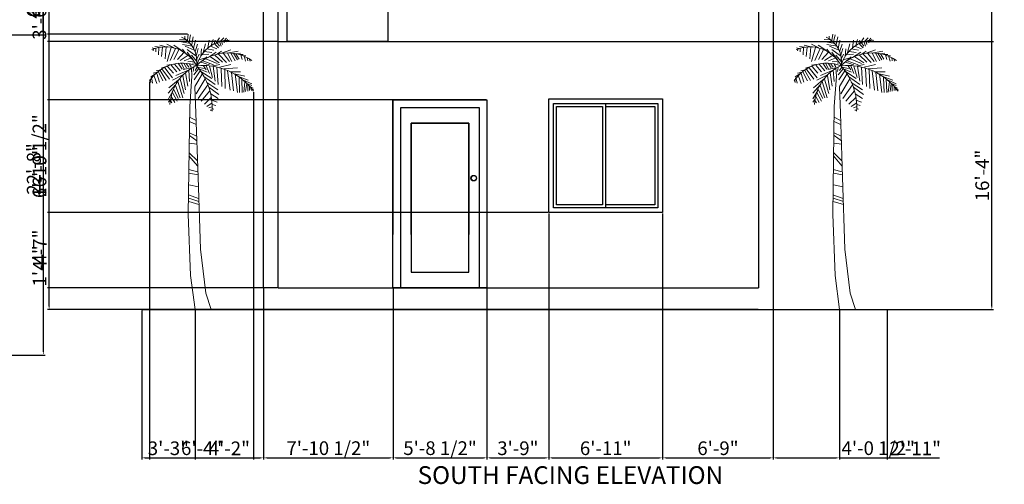
# Model space of a CAD drawing. Units: inches. Extents: x 1344 to 2521, y 3236 to 4924.
# Tile 13 of 14: x 1801 to 2521, y 4059 to 4398. Entities that reach past the tile are written whole.
import ezdxf

# ---------------------------------------------------------------- set-up
doc = ezdxf.new("R2010")
doc.units = ezdxf.units.IN
for name, color, linetype, lineweight in [('A-ANNO-DIMS', 2, 'Continuous', 18), ('A-ANNO-TEXT', 7, 'Continuous', 25), ('A-DOOR', 50, 'Continuous', 25), ('A-ELEV', 7, 'Continuous', 25), ('A-GLAZ', 150, 'Continuous', 25), ('L-PLNT', 82, 'Continuous', 13)]:
    doc.layers.add(name, color=color, linetype=linetype, lineweight=lineweight)
doc.styles.get("Standard").update_dxf_attribs({"font": 'arial.ttf'})
doc.dimstyles.new('ISO-25', dxfattribs={"dimtxt": 10, "dimasz": 2.5, "dimexe": 1.25, "dimexo": 0.625, "dimtad": 1, "dimdec": 0, "dimlunit": 4, "dimtxsty": 'Standard', "dimcen": 2.5, "dimadec": 0, "dimazin": 0, "dimtfac": 1, "dimtdec": 0, "dimtmove": 0, "dimatfit": 3, "dimfxl": 1, "dimarcsym": 0})

# ---------------------------------------------------------------- blocks, each defined once
blk = doc.blocks.new('*U10')
for p, q in [((1.5, 1.5), (1.5, 34.5)), ((1.5, 34.5), (18, 34.5)), ((18, 1.5), (18, 34.5)), ((18, 34.5), (34.5, 34.5)), ((34.5, 34.5), (34.5, 1.5)), ((18, 1.5), (1.5, 1.5)), ((34.5, 1.5), (18, 1.5))]:
    blk.add_line(p, q)
blk.add_lwpolyline([(0, 0), (0, 36), (36, 36), (36, 0)], close=True)
for points in [[(17, 33.5), (17, 2.5), (2.5, 2.5), (2.5, 33.5), (17, 33.5)], [(18, 33.5), (33.5, 33.5), (33.5, 2.5), (18, 2.5)]]:
    blk.add_lwpolyline(points)
blk = doc.blocks.new('*U13')
blk.add_lwpolyline([(3.12, 0.01), (0.12, 0.01), (0.12, 72.01), (36.12, 72.01), (36.12, 0.01), (33.12, 0.01)])
for points in [[(33.12, 68.99), (33.12, 0.01), (3.12, 0.01), (3.12, 68.99)], [(29.12, 6.01), (29.12, 62.99), (7.12, 62.99), (7.12, 6.01)]]:
    blk.add_lwpolyline(points, close=True)
blk.add_circle((31.12, 42.01), 1)
blk = doc.blocks.new('*U14')
for p, q in [((-6.727, 197.202), (-11.366, 197.45)), ((-3.441, 194.477), (-10.013, 195.716)), ((-7.5, 199.68), (-7.5, 197.946)), ((-5.567, 196.707), (-4.987, 201.167)), ((-4.407, 195.716), (-3.247, 200.672)), ((-2.474, 193.733), (-1.315, 199.433)), ((-1.121, 190.759), (0.232, 196.955)), ((9.317, 191.255), (10.283, 196.955)), ((11.829, 192.99), (13.182, 197.45)), ((13.956, 194.229), (14.729, 196.955)), ((15.116, 194.477), (17.822, 198.689)), ((16.082, 194.972), (17.822, 192.494)), ((18.015, 195.716), (20.914, 198.689)), ((18.015, 195.468), (18.981, 192.494)), ((19.368, 196.459), (19.948, 193.733)), ((20.914, 196.459), (21.301, 194.972)), ((21.301, 196.459), (22.847, 198.441)), ((22.074, 196.707), (23.427, 195.716)), ((23.234, 196.707), (23.62, 197.698)), ((-29.729, 190.759), (-31.469, 191.255)), ((-30.309, 190.512), (-30.695, 189.025)), ((-25.283, 191.751), (-29.342, 192.246)), ((-28.763, 190.759), (-28.763, 188.281)), ((-26.443, 191.503), (-26.636, 186.051)), ((-20.064, 191.751), (-25.863, 193.238)), ((-23.737, 191.751), (-24.51, 185.06)), ((-21.031, 191.998), (-21.804, 183.325)), ((-15.232, 191.255), (-20.644, 193.981)), ((-17.551, 191.503), (-20.451, 181.343)), ((-14.265, 190.759), (-18.131, 182.086)), ((-9.433, 189.025), (-15.618, 193.238)), ((-11.753, 189.768), (-15.425, 182.83)), ((-8.08, 188.034), (-12.912, 182.83)), ((-1.894, 192.494), (-9.24, 193.733)), ((-6.147, 186.299), (-9.24, 190.264)), ((-0.541, 189.52), (-7.307, 192.494)), ((-5.76, 190.016), (0.618, 185.308)), ((-5.76, 188.034), (-1.508, 182.582)), ((0.038, 188.281), (1.778, 193.981)), ((1.005, 185.803), (2.358, 190.759)), ((4.098, 185.06), (4.678, 190.512)), ((5.837, 187.786), (7.577, 194.229)), ((6.997, 188.529), (12.216, 187.786)), ((8.544, 190.512), (13.763, 189.52)), ((9.51, 184.317), (15.502, 188.034)), ((11.25, 192.494), (15.889, 190.512)), ((14.536, 193.981), (17.242, 191.255)), ((15.695, 186.299), (19.368, 188.777)), ((19.368, 187.29), (26.133, 189.768)), ((23.814, 187.29), (26.907, 181.343)), ((24.78, 187.538), (31.546, 188.777)), ((26.133, 187.29), (29.419, 181.838)), ((28.066, 187.29), (30.966, 182.582)), ((29.999, 186.795), (33.092, 187.29)), ((-12.332, 180.104), (-9.433, 175.643)), ((-4.987, 185.803), (-10.979, 182.086)), ((-10.206, 180.104), (-8.08, 175.891)), ((-8.273, 180.104), (-6.147, 176.635)), ((-3.247, 183.821), (-8.08, 181.838)), ((-1.315, 181.591), (-5.374, 181.095)), ((-2.668, 185.803), (1.198, 181.343)), ((-0.348, 180.352), (-1.894, 180.104)), ((1.005, 182.582), (2.938, 186.547)), ((2.938, 182.582), (6.61, 183.821)), ((4.098, 180.847), (8.35, 179.608)), ((4.871, 186.051), (10.09, 186.547)), ((4.871, 181.591), (8.544, 184.812)), ((5.644, 181.838), (13.569, 178.865)), ((7.77, 183.325), (16.082, 179.856)), ((11.25, 184.812), (17.628, 180.352)), ((14.536, 185.803), (19.948, 180.847)), ((17.242, 186.547), (23.041, 180.599)), ((20.721, 187.042), (25.167, 181.343)), ((29.806, 186.795), (32.319, 183.078)), ((32.512, 186.299), (35.218, 186.299)), ((33.479, 186.051), (34.445, 182.83)), ((35.605, 185.556), (37.151, 185.308)), ((35.798, 185.308), (36.958, 181.591)), ((38.118, 184.317), (38.504, 181.838)), ((39.857, 182.83), (40.244, 181.591)), ((-27.409, 173.413), (-30.695, 172.67)), ((-25.09, 175.148), (-28.376, 174.404)), ((-26.829, 173.661), (-23.544, 167.218)), ((-25.476, 174.652), (-21.224, 167.466)), ((-21.031, 177.626), (-24.897, 176.387)), ((-24.317, 175.891), (-18.711, 168.457)), ((-22.191, 176.635), (-16.391, 169.448)), ((-15.618, 179.36), (-20.644, 178.617)), ((-20.064, 177.626), (-15.812, 172.67)), ((-17.358, 178.617), (-13.299, 173.661)), ((-15.038, 179.36), (-10.786, 174.404)), ((-4.214, 175.148), (-14.072, 170.935)), ((-1.701, 176.882), (-8.66, 175.396)), ((-6.92, 172.917), (-5.374, 163.253)), ((-6.34, 179.608), (-4.6, 177.13)), ((-4.6, 174.9), (-4.021, 166.722)), ((-4.021, 179.36), (-2.861, 177.378)), ((-2.668, 176.387), (-2.376, 170.594)), ((-0.928, 176.882), (-1.508, 173.909)), ((2.551, 175.891), (-0.928, 171.431)), ((3.711, 174.404), (-0.541, 167.961)), ((1.585, 177.13), (0.038, 174.652)), ((1.585, 177.13), (6.61, 176.139)), ((2.938, 175.891), (8.737, 173.413)), ((4.291, 173.909), (12.216, 168.953)), ((6.224, 178.121), (8.157, 175.148)), ((7.384, 178.369), (10.476, 179.36)), ((8.157, 178.121), (10.476, 172.422)), ((10.476, 177.874), (12.796, 169.696)), ((11.829, 177.874), (18.015, 179.113)), ((13.182, 177.874), (14.729, 166.97)), ((15.889, 177.13), (16.855, 164.492)), ((18.015, 177.13), (26.133, 179.113)), ((18.981, 175.891), (19.561, 163.005)), ((20.914, 175.891), (30.966, 176.635)), ((21.688, 175.396), (22.074, 161.518)), ((23.814, 174.404), (25.554, 160.279)), ((25.554, 173.661), (33.285, 173.661)), ((26.52, 173.165), (28.066, 159.784)), ((-32.628, 167.961), (-33.208, 167.961)), ((-32.628, 167.713), (-32.435, 165.979)), ((-28.956, 172.174), (-32.435, 170.192)), ((-31.082, 169.944), (-32.435, 169.2)), ((-31.662, 168.705), (-31.082, 165.483)), ((-29.922, 170.687), (-27.989, 165.235)), ((-27.989, 172.422), (-26.056, 166.227)), ((-12.139, 167.961), (-19.098, 162.014)), ((-8.466, 171.678), (-16.585, 167.713)), ((-12.719, 166.722), (-9.046, 154.828)), ((-10.979, 168.457), (-7.887, 157.801)), ((-8.853, 170.935), (-7.113, 160.527)), ((5.257, 171.926), (-0.155, 163.005)), ((7.384, 168.705), (0.812, 157.553)), ((6.417, 170.439), (14.729, 164.492)), ((8.544, 165.979), (16.662, 160.527)), ((28.839, 172.174), (36.378, 170.687)), ((29.226, 171.926), (30.966, 158.545)), ((30.966, 170.687), (38.891, 167.713)), ((32.126, 169.696), (32.512, 158.545)), ((34.058, 168.705), (34.445, 158.545)), ((35.412, 167.713), (41.404, 164.988)), ((36.378, 166.474), (35.605, 158.792)), ((-14.265, 164.244), (-19.678, 158.049)), ((-16.005, 160.031), (-19.484, 154.084)), ((-16.585, 158.545), (-13.106, 152.35)), ((-15.618, 160.775), (-12.332, 154.332)), ((-14.265, 163.749), (-10.786, 154.828)), ((9.317, 164.244), (2.358, 154.332)), ((10.863, 159.784), (4.484, 152.35)), ((10.09, 162.51), (17.435, 157.058)), ((37.731, 165.235), (36.958, 159.288)), ((37.924, 165.235), (41.404, 163.749)), ((38.504, 164.492), (38.504, 159.536)), ((39.664, 163.253), (42.37, 161.766)), ((39.857, 162.757), (39.857, 160.031)), ((40.824, 161.766), (41.21, 160.031)), ((41.21, 161.518), (42.757, 160.279)), ((-18.131, 153.589), (-19.484, 151.606)), ((-17.938, 152.597), (-16.972, 151.111)), ((-17.358, 155.819), (-14.845, 151.358)), ((11.829, 155.075), (6.804, 150.119)), ((11.443, 157.553), (16.855, 154.332)), ((12.216, 153.093), (16.082, 151.606)), ((12.603, 151.111), (8.544, 148.385)), ((12.216, 148.137), (10.09, 147.393)), ((12.409, 145.659), (11.056, 145.659)), ((12.409, 146.898), (13.763, 146.402)), ((12.603, 149.872), (15.116, 149.128)), ((-4.081, 140.645), (0.753, 138.261)), ((-4.081, 137.547), (0.753, 135.163)), ((-4.081, 129.205), (1.124, 126.821)), ((-4.081, 127.298), (1.31, 123.246)), ((-4.081, 121.578), (1.31, 120.863)), ((-4.453, 112.283), (1.682, 105.133)), ((-4.267, 114.428), (1.682, 108.708)), ((-4.639, 102.273), (1.868, 100.604)), ((-4.453, 99.651), (2.24, 98.459)), ((-4.453, 91.071), (2.426, 89.641)), ((-4.825, 83.921), (2.612, 81.061)), ((-4.639, 81.299), (2.797, 78.916)), ((-4.639, 78.916), (2.797, 76.771))]:
    blk.add_line(p, q)
for points in [[(-2.363, 170.553), (-3.88, 148.505), (-4.988, 69.634), (-3.325, 24.869), (0, 0)], [(-0.116, 162.848), (0.554, 143.532), (2.217, 96.635), (3.88, 44.054), (7.76, 12.079), (11.64, 0)]]:
    blk.add_lwpolyline(points)
for centre, radius, start, end in [((-18.427, 181.448), 19.715, 350.285, 64.11229), ((25.595, 171.567), 25.395, 91.40319, 163.882), ((-21.738, 166.094), 25.899, 27.67115, 112.5305), ((23.687, 155.341), 32.188, 56.19272, 134.3213), ((-9.259, 151.732), 28.386, 68.38311, 147.5322), ((14.394, 148.393), 32.752, 113.7592, 177.4133), ((5.828, 132.718), 45.639, 35.98777, 95.82273), ((-32.8, 147.923), 45.309, 356.1943, 41.37848)]:
    blk.add_arc(centre, radius, start, end)
blk = doc.blocks.new('*D89')
at = {"layer": 'A-ANNO-DIMS', "color": 0, "lineweight": -2, "transparency": 16777216}
for p, q in [((1774.14, 4425.27), (1820.02, 4425.27)), ((1818.77, 4422.77), (1818.77, 4155.71)), ((1774.14, 4153.21), (1820.02, 4153.21))]:
    blk.add_line(p, q, dxfattribs=at)
at = {"layer": 'A-ANNO-DIMS', "color": 0, "lineweight": 100, "transparency": 16777216}
for points in [[(1818.35, 4422.77), (1819.18, 4422.77), (1818.77, 4425.27)], [(1818.35, 4155.71), (1819.18, 4155.71), (1818.77, 4153.21)]]:
    blk.add_solid(points, dxfattribs=at)
at = {"layer": 'Defpoints', "color": 0, "lineweight": 100, "transparency": 16777216}
for p in [(1773.52, 4425.27), (1773.52, 4153.21), (1818.77, 4153.21)]:
    blk.add_point(p, dxfattribs=at)
at = {"layer": 'A-ANNO-DIMS', "color": 0, "transparency": 16777216, "insert": (1813.04, 4289.24), "char_height": 10, "attachment_point": 5, "rotation": 90}
blk.add_mtext('22\'-8"', dxfattribs=at)
blk = doc.blocks.new('*D98')
at = {"layer": 'A-ANNO-DIMS', "color": 0, "lineweight": -2, "transparency": 16777216}
for p, q in [((1562.2, 4466.57), (1820.02, 4466.57)), ((1818.77, 4464.07), (1818.77, 4389.64)), ((1562.2, 4387.14), (1820.02, 4387.14))]:
    blk.add_line(p, q, dxfattribs=at)
at = {"layer": 'A-ANNO-DIMS', "color": 0, "lineweight": 100, "transparency": 16777216}
for points in [[(1818.35, 4464.07), (1819.18, 4464.07), (1818.77, 4466.57)], [(1818.35, 4389.64), (1819.18, 4389.64), (1818.77, 4387.14)]]:
    blk.add_solid(points, dxfattribs=at)
at = {"layer": 'Defpoints', "color": 0, "lineweight": 100, "transparency": 16777216}
for p in [(1561.57, 4466.57), (1561.57, 4387.14), (1818.77, 4387.14)]:
    blk.add_point(p, dxfattribs=at)
at = {"layer": 'A-ANNO-DIMS', "color": 0, "transparency": 16777216, "insert": (1812.97, 4426.85), "char_height": 10, "attachment_point": 5, "rotation": 90}
blk.add_mtext('6\'-7 1/2"', dxfattribs=at)
blk = doc.blocks.new('*D103')
at = {"layer": 'A-ANNO-DIMS', "color": 0, "lineweight": -2, "transparency": 16777216}
for p, q in [((1729.14, 4441.19), (1820.02, 4441.19)), ((1818.77, 4389.64), (1818.77, 4438.69)), ((1729.14, 4387.14), (1820.02, 4387.14))]:
    blk.add_line(p, q, dxfattribs=at)
at = {"layer": 'A-ANNO-DIMS', "color": 0, "lineweight": 100, "transparency": 16777216}
for points in [[(1818.35, 4438.69), (1819.18, 4438.69), (1818.77, 4441.19)], [(1818.35, 4389.64), (1819.18, 4389.64), (1818.77, 4387.14)]]:
    blk.add_solid(points, dxfattribs=at)
at = {"layer": 'Defpoints', "color": 0, "lineweight": 100, "transparency": 16777216}
for p in [(1728.52, 4441.19), (1818.77, 4441.19), (1728.52, 4387.14)]:
    blk.add_point(p, dxfattribs=at)
at = {"layer": 'A-ANNO-DIMS', "color": 0, "transparency": 16777216, "insert": (1813.04, 4414.17), "char_height": 10, "attachment_point": 5, "rotation": 90}
blk.add_mtext('4\'-6"', dxfattribs=at)
blk = doc.blocks.new('*D124')
at = {"layer": 'A-ANNO-DIMS', "color": 0, "lineweight": -2, "transparency": 16777216}
for p, q in [((2074.33, 4201.82), (2074.33, 4076.85)), ((1979.76, 4185.86), (1979.76, 4076.85)), ((1982.26, 4078.1), (2071.83, 4078.1))]:
    blk.add_line(p, q, dxfattribs=at)
at = {"layer": 'A-ANNO-DIMS', "color": 0, "lineweight": 100, "transparency": 16777216}
for points in [[(1982.26, 4078.51), (1982.26, 4077.68), (1979.76, 4078.1)], [(2071.83, 4078.51), (2071.83, 4077.68), (2074.33, 4078.1)]]:
    blk.add_solid(points, dxfattribs=at)
at = {"layer": 'Defpoints', "color": 0, "lineweight": 100, "transparency": 16777216}
for p in [(2074.33, 4202.45), (1979.76, 4186.48), (2074.33, 4078.1)]:
    blk.add_point(p, dxfattribs=at)
at = {"layer": 'A-ANNO-DIMS', "color": 0, "transparency": 16777216, "insert": (2027.05, 4083.89), "char_height": 10, "attachment_point": 5}
blk.add_mtext('7\'-10 1/2"', dxfattribs=at)
blk = doc.blocks.new('*D125')
at = {"layer": 'A-ANNO-DIMS', "color": 0, "lineweight": -2, "transparency": 16777216}
for p, q in [((2074.33, 4201.82), (2074.33, 4076.85)), ((2143.01, 4201.82), (2143.01, 4076.85)), ((2076.83, 4078.1), (2140.51, 4078.1))]:
    blk.add_line(p, q, dxfattribs=at)
at = {"layer": 'A-ANNO-DIMS', "color": 0, "lineweight": 100, "transparency": 16777216}
for points in [[(2076.83, 4078.51), (2076.83, 4077.68), (2074.33, 4078.1)], [(2140.51, 4078.51), (2140.51, 4077.68), (2143.01, 4078.1)]]:
    blk.add_solid(points, dxfattribs=at)
at = {"layer": 'Defpoints', "color": 0, "lineweight": 100, "transparency": 16777216}
for p in [(2074.33, 4202.45), (2143.01, 4202.45), (2143.01, 4078.1)]:
    blk.add_point(p, dxfattribs=at)
at = {"layer": 'A-ANNO-DIMS', "color": 0, "transparency": 16777216, "insert": (2108.67, 4083.89), "char_height": 10, "attachment_point": 5}
blk.add_mtext('5\'-8 1/2"', dxfattribs=at)
blk = doc.blocks.new('*D126')
at = {"layer": 'A-ANNO-DIMS', "color": 0, "lineweight": -2, "transparency": 16777216}
for p, q in [((2188.14, 4256.71), (2188.14, 4076.85)), ((2143.01, 4201.82), (2143.01, 4076.85)), ((2145.51, 4078.1), (2185.64, 4078.1))]:
    blk.add_line(p, q, dxfattribs=at)
at = {"layer": 'A-ANNO-DIMS', "color": 0, "lineweight": 100, "transparency": 16777216}
for points in [[(2145.51, 4078.51), (2145.51, 4077.68), (2143.01, 4078.1)], [(2185.64, 4078.51), (2185.64, 4077.68), (2188.14, 4078.1)]]:
    blk.add_solid(points, dxfattribs=at)
at = {"layer": 'Defpoints', "color": 0, "lineweight": 100, "transparency": 16777216}
for p in [(2188.14, 4257.33), (2143.01, 4202.45), (2188.14, 4078.1)]:
    blk.add_point(p, dxfattribs=at)
at = {"layer": 'A-ANNO-DIMS', "color": 0, "transparency": 16777216, "insert": (2165.57, 4083.83), "char_height": 10, "attachment_point": 5}
blk.add_mtext('3\'-9"', dxfattribs=at)
blk = doc.blocks.new('*D127')
at = {"layer": 'A-ANNO-DIMS', "color": 0, "lineweight": -2, "transparency": 16777216}
for p, q in [((2188.14, 4256.71), (2188.14, 4076.85)), ((2271.38, 4256.71), (2271.38, 4076.85)), ((2190.64, 4078.1), (2268.88, 4078.1))]:
    blk.add_line(p, q, dxfattribs=at)
at = {"layer": 'A-ANNO-DIMS', "color": 0, "lineweight": 100, "transparency": 16777216}
for points in [[(2190.64, 4078.51), (2190.64, 4077.68), (2188.14, 4078.1)], [(2268.88, 4078.51), (2268.88, 4077.68), (2271.38, 4078.1)]]:
    blk.add_solid(points, dxfattribs=at)
at = {"layer": 'Defpoints', "color": 0, "lineweight": 100, "transparency": 16777216}
for p in [(2188.14, 4257.33), (2271.38, 4257.33), (2271.38, 4078.1)]:
    blk.add_point(p, dxfattribs=at)
at = {"layer": 'A-ANNO-DIMS', "color": 0, "transparency": 16777216, "insert": (2229.76, 4083.83), "char_height": 10, "attachment_point": 5}
blk.add_mtext('6\'-11"', dxfattribs=at)
blk = doc.blocks.new('*D128')
at = {"layer": 'A-ANNO-DIMS', "color": 0, "lineweight": -2, "transparency": 16777216}
for p, q in [((2271.38, 4256.71), (2271.38, 4076.85)), ((2352.24, 4185.86), (2352.24, 4076.85)), ((2273.88, 4078.1), (2349.74, 4078.1))]:
    blk.add_line(p, q, dxfattribs=at)
at = {"layer": 'A-ANNO-DIMS', "color": 0, "lineweight": 100, "transparency": 16777216}
for points in [[(2273.88, 4078.51), (2273.88, 4077.68), (2271.38, 4078.1)], [(2349.74, 4078.51), (2349.74, 4077.68), (2352.24, 4078.1)]]:
    blk.add_solid(points, dxfattribs=at)
at = {"layer": 'Defpoints', "color": 0, "lineweight": 100, "transparency": 16777216}
for p in [(2271.38, 4257.33), (2352.24, 4186.48), (2352.24, 4078.1)]:
    blk.add_point(p, dxfattribs=at)
at = {"layer": 'A-ANNO-DIMS', "color": 0, "transparency": 16777216, "insert": (2311.81, 4083.83), "char_height": 10, "attachment_point": 5}
blk.add_mtext('6\'-9"', dxfattribs=at)
blk = doc.blocks.new('*D129')
at = {"layer": 'A-ANNO-DIMS', "color": 0, "lineweight": -2, "transparency": 16777216}
for p, q in [((1890.65, 4185.86), (1890.65, 4076.85)), ((1929.67, 4185.86), (1929.67, 4076.85)), ((1893.15, 4078.1), (1927.17, 4078.1))]:
    blk.add_line(p, q, dxfattribs=at)
at = {"layer": 'A-ANNO-DIMS', "color": 0, "lineweight": 100, "transparency": 16777216}
for points in [[(1893.15, 4078.51), (1893.15, 4077.68), (1890.65, 4078.1)], [(1927.17, 4078.51), (1927.17, 4077.68), (1929.67, 4078.1)]]:
    blk.add_solid(points, dxfattribs=at)
at = {"layer": 'Defpoints', "color": 0, "lineweight": 100, "transparency": 16777216}
for p in [(1890.65, 4186.48), (1929.67, 4186.48), (1929.67, 4078.1)]:
    blk.add_point(p, dxfattribs=at)
at = {"layer": 'A-ANNO-DIMS', "color": 0, "transparency": 16777216, "insert": (1910.16, 4083.83), "char_height": 10, "attachment_point": 5}
blk.add_mtext('3\'-3"', dxfattribs=at)
blk = doc.blocks.new('*D130')
at = {"layer": 'A-ANNO-DIMS', "color": 0, "lineweight": -2, "transparency": 16777216}
for p, q in [((1929.67, 4185.86), (1929.67, 4076.85)), ((1979.76, 4185.86), (1979.76, 4076.85)), ((1932.17, 4078.1), (1977.26, 4078.1))]:
    blk.add_line(p, q, dxfattribs=at)
at = {"layer": 'A-ANNO-DIMS', "color": 0, "lineweight": 100, "transparency": 16777216}
for points in [[(1932.17, 4078.51), (1932.17, 4077.68), (1929.67, 4078.1)], [(1977.26, 4078.51), (1977.26, 4077.68), (1979.76, 4078.1)]]:
    blk.add_solid(points, dxfattribs=at)
at = {"layer": 'Defpoints', "color": 0, "lineweight": 100, "transparency": 16777216}
for p in [(1929.67, 4186.48), (1979.76, 4186.48), (1979.76, 4078.1)]:
    blk.add_point(p, dxfattribs=at)
at = {"layer": 'A-ANNO-DIMS', "color": 0, "transparency": 16777216, "insert": (1954.72, 4083.74), "char_height": 10, "attachment_point": 5}
blk.add_mtext('4\'-2"', dxfattribs=at)
blk = doc.blocks.new('*D131')
at = {"layer": 'A-ANNO-DIMS', "color": 0, "lineweight": -2, "transparency": 16777216}
for p, q in [((2352.24, 4185.86), (2352.24, 4076.85)), ((2400.71, 4185.86), (2400.71, 4076.85)), ((2354.74, 4078.1), (2398.21, 4078.1)), ((2400.71, 4078.1), (2454.74, 4078.1))]:
    blk.add_line(p, q, dxfattribs=at)
at = {"layer": 'A-ANNO-DIMS', "color": 0, "lineweight": 100, "transparency": 16777216}
for points in [[(2354.74, 4078.51), (2354.74, 4077.68), (2352.24, 4078.1)], [(2398.21, 4078.51), (2398.21, 4077.68), (2400.71, 4078.1)]]:
    blk.add_solid(points, dxfattribs=at)
at = {"layer": 'Defpoints', "color": 0, "lineweight": 100, "transparency": 16777216}
for p in [(2352.24, 4186.48), (2400.71, 4186.48), (2400.71, 4078.1)]:
    blk.add_point(p, dxfattribs=at)
at = {"layer": 'A-ANNO-DIMS', "color": 0, "transparency": 16777216, "insert": (2428.97, 4083.89), "char_height": 10, "attachment_point": 5}
blk.add_mtext('4\'-0 1/2"', dxfattribs=at)
blk = doc.blocks.new('*D132')
at = {"layer": 'A-ANNO-DIMS', "color": 0, "lineweight": -2, "transparency": 16777216}
for p, q in [((2400.71, 4185.86), (2400.71, 4076.85)), ((2435.55, 4185.86), (2435.55, 4076.85)), ((2403.21, 4078.1), (2433.05, 4078.1)), ((2435.55, 4078.1), (2473.83, 4078.1))]:
    blk.add_line(p, q, dxfattribs=at)
at = {"layer": 'A-ANNO-DIMS', "color": 0, "lineweight": 100, "transparency": 16777216}
for points in [[(2403.21, 4078.51), (2403.21, 4077.68), (2400.71, 4078.1)], [(2433.05, 4078.51), (2433.05, 4077.68), (2435.55, 4078.1)]]:
    blk.add_solid(points, dxfattribs=at)
at = {"layer": 'Defpoints', "color": 0, "lineweight": 100, "transparency": 16777216}
for p in [(2400.71, 4186.48), (2435.55, 4186.48), (2435.55, 4078.1)]:
    blk.add_point(p, dxfattribs=at)
at = {"layer": 'A-ANNO-DIMS', "color": 0, "transparency": 16777216, "insert": (2455.94, 4083.74), "char_height": 10, "attachment_point": 5}
blk.add_mtext('2\'-11"', dxfattribs=at)
blk = doc.blocks.new('*D133')
at = {"layer": 'A-ANNO-DIMS', "color": 0, "lineweight": -2, "transparency": 16777216}
for p, q in [((1924.06, 4387.65), (1821.78, 4387.65)), ((1823.03, 4188.98), (1823.03, 4385.15)), ((1890.03, 4186.48), (1821.78, 4186.48))]:
    blk.add_line(p, q, dxfattribs=at)
at = {"layer": 'A-ANNO-DIMS', "color": 0, "lineweight": 100, "transparency": 16777216}
for points in [[(1822.61, 4385.15), (1823.44, 4385.15), (1823.03, 4387.65)], [(1822.61, 4188.98), (1823.44, 4188.98), (1823.03, 4186.48)]]:
    blk.add_solid(points, dxfattribs=at)
at = {"layer": 'Defpoints', "color": 0, "lineweight": 100, "transparency": 16777216}
for p in [(1823.03, 4387.65), (1924.68, 4387.65), (1890.65, 4186.48)]:
    blk.add_point(p, dxfattribs=at)
at = {"layer": 'A-ANNO-DIMS', "color": 0, "transparency": 16777216, "insert": (1817.29, 4287.07), "char_height": 10, "attachment_point": 5, "rotation": 90}
blk.add_mtext('16\'-9"', dxfattribs=at)
blk = doc.blocks.new('*D134')
at = {"layer": 'A-ANNO-DIMS', "color": 0, "lineweight": -2, "transparency": 16777216}
for p, q in [((1896.46, 4352.83), (1896.46, 4076.85)), ((1972.43, 4345.39), (1972.43, 4076.85)), ((1898.96, 4078.1), (1969.93, 4078.1))]:
    blk.add_line(p, q, dxfattribs=at)
at = {"layer": 'A-ANNO-DIMS', "color": 0, "lineweight": 100, "transparency": 16777216}
for points in [[(1898.96, 4078.51), (1898.96, 4077.68), (1896.46, 4078.1)], [(1969.93, 4078.51), (1969.93, 4077.68), (1972.43, 4078.1)]]:
    blk.add_solid(points, dxfattribs=at)
at = {"layer": 'Defpoints', "color": 0, "lineweight": 100, "transparency": 16777216}
for p in [(1896.46, 4353.45), (1972.43, 4346.02), (1972.43, 4078.1)]:
    blk.add_point(p, dxfattribs=at)
at = {"layer": 'A-ANNO-DIMS', "color": 0, "transparency": 16777216, "insert": (1934.45, 4083.83), "char_height": 10, "attachment_point": 5}
blk.add_mtext('6\'-4"', dxfattribs=at)
blk = doc.blocks.new('*D135')
at = {"layer": 'A-ANNO-DIMS', "color": 0, "lineweight": -2, "transparency": 16777216}
for p, q in [((2342.13, 4382.45), (2513.22, 4382.45)), ((2511.97, 4188.98), (2511.97, 4379.95)), ((2352.87, 4186.48), (2513.22, 4186.48))]:
    blk.add_line(p, q, dxfattribs=at)
at = {"layer": 'A-ANNO-DIMS', "color": 0, "lineweight": 100, "transparency": 16777216}
for points in [[(2511.56, 4379.95), (2512.39, 4379.95), (2511.97, 4382.45)], [(2511.56, 4188.98), (2512.39, 4188.98), (2511.97, 4186.48)]]:
    blk.add_solid(points, dxfattribs=at)
at = {"layer": 'Defpoints', "color": 0, "lineweight": 100, "transparency": 16777216}
for p in [(2341.5, 4382.45), (2511.97, 4382.45), (2352.24, 4186.48)]:
    blk.add_point(p, dxfattribs=at)
at = {"layer": 'A-ANNO-DIMS', "color": 0, "transparency": 16777216, "insert": (2506.24, 4284.46), "char_height": 10, "attachment_point": 5, "rotation": 90}
blk.add_mtext('16\'-4"', dxfattribs=at)
blk = doc.blocks.new('*D136')
at = {"layer": 'A-ANNO-DIMS', "color": 0, "lineweight": -2, "transparency": 16777216}
for p, q in [((2342.13, 4562.45), (2513.22, 4562.45)), ((2511.97, 4384.95), (2511.97, 4559.95)), ((2342.13, 4382.45), (2513.22, 4382.45))]:
    blk.add_line(p, q, dxfattribs=at)
at = {"layer": 'A-ANNO-DIMS', "color": 0, "lineweight": 100, "transparency": 16777216}
for points in [[(2511.56, 4559.95), (2512.39, 4559.95), (2511.97, 4562.45)], [(2511.56, 4384.95), (2512.39, 4384.95), (2511.97, 4382.45)]]:
    blk.add_solid(points, dxfattribs=at)
at = {"layer": 'Defpoints', "color": 0, "lineweight": 100, "transparency": 16777216}
for p in [(2341.5, 4562.45), (2511.97, 4562.45), (2341.5, 4382.45)]:
    blk.add_point(p, dxfattribs=at)
at = {"layer": 'A-ANNO-DIMS', "color": 0, "transparency": 16777216, "insert": (2506.24, 4472.45), "char_height": 10, "attachment_point": 5, "rotation": 90}
blk.add_mtext('15\'-0"', dxfattribs=at)
blk = doc.blocks.new('*D138')
at = {"layer": 'A-ANNO-DIMS', "color": 0, "lineweight": -2, "transparency": 16777216}
for p, q in [((2352.87, 4753.19), (2513.22, 4753.19)), ((2511.97, 4188.98), (2511.97, 4750.69)), ((2352.87, 4186.48), (2513.22, 4186.48))]:
    blk.add_line(p, q, dxfattribs=at)
at = {"layer": 'A-ANNO-DIMS', "color": 0, "lineweight": 100, "transparency": 16777216}
for points in [[(2511.56, 4750.69), (2512.39, 4750.69), (2511.97, 4753.19)], [(2511.56, 4188.98), (2512.39, 4188.98), (2511.97, 4186.48)]]:
    blk.add_solid(points, dxfattribs=at)
at = {"layer": 'Defpoints', "color": 0, "lineweight": 100, "transparency": 16777216}
for p in [(2352.24, 4753.19), (2511.97, 4753.19), (2352.24, 4186.48)]:
    blk.add_point(p, dxfattribs=at)
at = {"layer": 'A-ANNO-DIMS', "color": 0, "transparency": 16777216, "insert": (2506.18, 4469.83), "char_height": 10, "attachment_point": 5, "rotation": 90}
blk.add_mtext('47\'-2 1/2"', dxfattribs=at)
blk = doc.blocks.new('*D139')
at = {"layer": 'A-ANNO-DIMS', "color": 0, "lineweight": -2, "transparency": 16777216}
for p, q in [((1823.03, 4202.45), (1823.03, 4231.84)), ((1989.88, 4202.45), (1821.78, 4202.45)), ((1823.03, 4188.98), (1823.03, 4199.95)), ((1979.14, 4186.48), (1821.78, 4186.48))]:
    blk.add_line(p, q, dxfattribs=at)
at = {"layer": 'A-ANNO-DIMS', "color": 0, "lineweight": 100, "transparency": 16777216}
for points in [[(1822.61, 4199.95), (1823.44, 4199.95), (1823.03, 4202.45)], [(1822.61, 4188.98), (1823.44, 4188.98), (1823.03, 4186.48)]]:
    blk.add_solid(points, dxfattribs=at)
at = {"layer": 'Defpoints', "color": 0, "lineweight": 100, "transparency": 16777216}
for p in [(1823.03, 4202.45), (1990.5, 4202.45), (1979.76, 4186.48)]:
    blk.add_point(p, dxfattribs=at)
at = {"layer": 'A-ANNO-DIMS', "color": 0, "transparency": 16777216, "insert": (1817.38, 4218.39), "char_height": 10, "attachment_point": 5, "rotation": 90}
blk.add_mtext('1\'-4"', dxfattribs=at)
blk = doc.blocks.new('*D140')
at = {"layer": 'A-ANNO-DIMS', "color": 0, "lineweight": -2, "transparency": 16777216}
for p, q in [((2187.52, 4257.33), (1821.78, 4257.33)), ((1823.03, 4204.95), (1823.03, 4254.83)), ((1989.88, 4202.45), (1821.78, 4202.45))]:
    blk.add_line(p, q, dxfattribs=at)
at = {"layer": 'A-ANNO-DIMS', "color": 0, "lineweight": 100, "transparency": 16777216}
for points in [[(1822.61, 4254.83), (1823.44, 4254.83), (1823.03, 4257.33)], [(1822.61, 4204.95), (1823.44, 4204.95), (1823.03, 4202.45)]]:
    blk.add_solid(points, dxfattribs=at)
at = {"layer": 'Defpoints', "color": 0, "lineweight": 100, "transparency": 16777216}
for p in [(1823.03, 4257.33), (2188.14, 4257.33), (1990.5, 4202.45)]:
    blk.add_point(p, dxfattribs=at)
at = {"layer": 'A-ANNO-DIMS', "color": 0, "transparency": 16777216, "insert": (1817.4, 4229.89), "char_height": 10, "attachment_point": 5, "rotation": 90}
blk.add_mtext('4\'-7"', dxfattribs=at)
blk = doc.blocks.new('*D141')
at = {"layer": 'A-ANNO-DIMS', "color": 0, "lineweight": -2, "transparency": 16777216}
for p, q in [((2142.38, 4339.8), (1821.78, 4339.8)), ((1823.03, 4259.83), (1823.03, 4337.3)), ((2187.52, 4257.33), (1821.78, 4257.33))]:
    blk.add_line(p, q, dxfattribs=at)
at = {"layer": 'A-ANNO-DIMS', "color": 0, "lineweight": 100, "transparency": 16777216}
for points in [[(1822.61, 4337.3), (1823.44, 4337.3), (1823.03, 4339.8)], [(1822.61, 4259.83), (1823.44, 4259.83), (1823.03, 4257.33)]]:
    blk.add_solid(points, dxfattribs=at)
at = {"layer": 'Defpoints', "color": 0, "lineweight": 100, "transparency": 16777216}
for p in [(1823.03, 4339.8), (2143.01, 4339.8), (2188.14, 4257.33)]:
    blk.add_point(p, dxfattribs=at)
at = {"layer": 'A-ANNO-DIMS', "color": 0, "transparency": 16777216, "insert": (1817.23, 4298.56), "char_height": 10, "attachment_point": 5, "rotation": 90}
blk.add_mtext('6\'-10 1/2"', dxfattribs=at)
blk = doc.blocks.new('*D142')
at = {"layer": 'A-ANNO-DIMS', "color": 0, "lineweight": -2, "transparency": 16777216}
for p, q in [((1823.03, 4382.45), (1823.03, 4436.07)), ((1989.88, 4382.45), (1821.78, 4382.45)), ((1823.03, 4342.3), (1823.03, 4379.95)), ((2142.38, 4339.8), (1821.78, 4339.8))]:
    blk.add_line(p, q, dxfattribs=at)
at = {"layer": 'A-ANNO-DIMS', "color": 0, "lineweight": 100, "transparency": 16777216}
for points in [[(1822.61, 4379.95), (1823.44, 4379.95), (1823.03, 4382.45)], [(1822.61, 4342.3), (1823.44, 4342.3), (1823.03, 4339.8)]]:
    blk.add_solid(points, dxfattribs=at)
at = {"layer": 'Defpoints', "color": 0, "lineweight": 100, "transparency": 16777216}
for p in [(1823.03, 4382.45), (1990.5, 4382.45), (2143.01, 4339.8)]:
    blk.add_point(p, dxfattribs=at)
at = {"layer": 'A-ANNO-DIMS', "color": 0, "transparency": 16777216, "insert": (1817.23, 4410.51), "char_height": 10, "attachment_point": 5, "rotation": 90}
blk.add_mtext('3\'-6 1/2"', dxfattribs=at)
blk = doc.blocks.new('*D143')
at = {"layer": 'A-ANNO-DIMS', "color": 0, "lineweight": -2, "transparency": 16777216}
for p, q in [((1823.03, 4405.88), (1823.03, 4466.34)), ((2080.18, 4405.88), (1821.78, 4405.88)), ((1823.03, 4384.95), (1823.03, 4403.38)), ((1989.88, 4382.45), (1821.78, 4382.45))]:
    blk.add_line(p, q, dxfattribs=at)
at = {"layer": 'A-ANNO-DIMS', "color": 0, "lineweight": 100, "transparency": 16777216}
for points in [[(1822.61, 4403.38), (1823.44, 4403.38), (1823.03, 4405.88)], [(1822.61, 4384.95), (1823.44, 4384.95), (1823.03, 4382.45)]]:
    blk.add_solid(points, dxfattribs=at)
at = {"layer": 'Defpoints', "color": 0, "lineweight": 100, "transparency": 16777216}
for p in [(1823.03, 4405.88), (2080.81, 4405.88), (1990.5, 4382.45)]:
    blk.add_point(p, dxfattribs=at)
at = {"layer": 'A-ANNO-DIMS', "color": 0, "transparency": 16777216, "insert": (1817.23, 4437.36), "char_height": 10, "attachment_point": 5, "rotation": 90}
blk.add_mtext('1\'-11 1/2"', dxfattribs=at)

msp = doc.modelspace()

# ---------------------------------------------------------------- linework, layer by layer
at = {"layer": 'A-ELEV'}
for p, q in [((1979.76, 4382.45), (1979.76, 4562.45)), ((1990.5, 4382.45), (1990.5, 4562.45)), ((2341.5, 4562.45), (2341.5, 4341.36)), ((2352.24, 4562.45), (2352.24, 4341.36)), ((1979.76, 4322.45), (1979.76, 4382.45)), ((1990.5, 4322.45), (1990.5, 4382.45)), ((1990.5, 4382.45), (2341.5, 4382.45)), ((2341.5, 4382.45), (2341.5, 4202.45)), ((2352.24, 4382.45), (2352.24, 4202.45)), ((1979.76, 4202.45), (1979.76, 4322.45)), ((1990.5, 4202.45), (1990.5, 4322.45)), ((1979.76, 4202.45), (1979.76, 4186.48)), ((1990.5, 4202.45), (2341.5, 4202.45)), ((1990.5, 4202.45), (2341.5, 4202.45)), ((2352.24, 4202.45), (2352.24, 4186.48)), ((1954.5, 4186.48), (1890.65, 4186.48)), ((1890.65, 4186.48), (2435.55, 4186.48)), ((1990.5, 4186.48), (1954.5, 4186.48)), ((2341.16, 4186.48), (2377.16, 4186.48))]:
    msp.add_line(p, q, dxfattribs=at)
msp.add_lwpolyline([(1996.97, 4732.77), (2070.56, 4732.77), (2070.56, 4382.45), (1996.97, 4382.45)], close=True, dxfattribs=at)
for points in [[(2074.33, 4241.36), (2074.33, 4339.8), (2143.01, 4339.8), (2143.01, 4241.36)], [(2080.05, 4241.36), (2080.05, 4334.03), (2137.28, 4334.03), (2137.28, 4241.36)], [(2087.68, 4241.36), (2087.68, 4322.58), (2129.65, 4322.58), (2129.65, 4241.36)], [(1990.5, 4202.45), (2341.16, 4202.45)], [(2341.16, 4186.48), (1990.5, 4186.48)]]:
    msp.add_lwpolyline(points, dxfattribs=at)
msp.add_circle((2133.31, 4282.52), 2.03, dxfattribs=at)

# ---------------------------------------------------------------- block references
at = {"layer": 'A-DOOR', "xscale": 1.907656361171789, "yscale": 1.907656361171789, "zscale": 1.907656361171789}
msp.add_blockref('*U13', (2074.09, 4202.42), dxfattribs=at)
at = {"layer": 'A-GLAZ', "xscale": 2.312102872961218, "yscale": 2.312102872961218, "zscale": 2.312102872961218}
msp.add_blockref('*U10', (2188.14, 4257.33), dxfattribs=at)
at = {"layer": 'L-PLNT'}
for p in [(1929.67, 4186.48), (2400.71, 4186.48)]:
    msp.add_blockref('*U14', p, dxfattribs=at)

# ---------------------------------------------------------------- texts
at = {"layer": 'A-ANNO-TEXT', "insert": (2092.3, 4071.99), "char_height": 12.9935, "attachment_point": 1}
msp.add_mtext_dynamic_manual_height_columns('SOUTH FACING ELEVATION', width=2122.9296, gutter_width=64.97, heights=[0], dxfattribs=at)

# ---------------------------------------------------------------- dimensions: what is measured, and where the dimension line sits
at = {"layer": 'A-ANNO-DIMS'}
for base, p1, p2, picture, middle in [((2511.97, 4753.19), (2352.24, 4186.48), (2352.24, 4753.19), '*D138', (2506.18, 4469.83)), ((2511.97, 4562.45), (2341.5, 4382.45), (2341.5, 4562.45), '*D136', (2506.24, 4472.45)), ((1818.77, 4387.14), (1561.57, 4466.57), (1561.57, 4387.14), '*D98', (1812.97, 4426.85)), ((1823.03, 4405.88), (1990.5, 4382.45), (2080.81, 4405.88), '*D143', (1817.23, 4437.36)), ((1818.7678, 4441.1901), (1728.5178, 4387.143), (1728.5178, 4441.1901), '*D103', (1813.0371, 4414.1665)), ((1823.0257, 4382.4452), (2143.0066, 4339.7965), (1990.5008, 4382.4452), '*D142', (1817.2267, 4410.5088)), ((1818.77, 4153.21), (1773.52, 4425.27), (1773.52, 4153.21), '*D89', (1813.04, 4289.24)), ((1823.03, 4387.65), (1890.65, 4186.48), (1924.68, 4387.65), '*D133', (1817.29, 4287.07)), ((2511.97, 4382.45), (2352.24, 4186.48), (2341.5, 4382.45), '*D135', (2506.24, 4284.46)), ((1823.03, 4339.8), (2188.14, 4257.33), (2143.01, 4339.8), '*D141', (1817.23, 4298.56)), ((1823.03, 4257.33), (1990.5, 4202.45), (2188.14, 4257.33), '*D140', (1817.4, 4229.89)), ((1823.03, 4202.45), (1979.76, 4186.48), (1990.5, 4202.45), '*D139', (1817.38, 4218.39))]:
    dim = msp.add_linear_dim(base=base, p1=p1, p2=p2, angle=90, dimstyle='ISO-25', override={"dimdec": 1, "dimlfac": 1, "dimrnd": 0, "dimzin": 1, "dimdsep": 46, "dimlunit": 4, "dimfrac": 2}, dxfattribs=at)
    dim.commit()
    dim.dimension.update_dxf_attribs({"geometry": picture, "text_midpoint": middle})
for base, p1, p2, picture, middle in [((1972.43, 4078.1), (1896.46, 4353.45), (1972.43, 4346.02), '*D134', (1934.45, 4083.83)), ((2188.14, 4078.1), (2143.01, 4202.45), (2188.14, 4257.33), '*D126', (2165.57, 4083.83)), ((2271.38, 4078.1), (2188.14, 4257.33), (2271.38, 4257.33), '*D127', (2229.76, 4083.83)), ((2352.24, 4078.1), (2271.38, 4257.33), (2352.24, 4186.48), '*D128', (2311.81, 4083.83)), ((2074.33, 4078.1), (1979.76, 4186.48), (2074.33, 4202.45), '*D124', (2027.05, 4083.89)), ((2143.01, 4078.1), (2074.33, 4202.45), (2143.01, 4202.45), '*D125', (2108.67, 4083.89)), ((1929.67, 4078.1), (1890.65, 4186.48), (1929.67, 4186.48), '*D129', (1910.16, 4083.83)), ((1979.76, 4078.1), (1929.67, 4186.48), (1979.76, 4186.48), '*D130', (1954.72, 4083.74)), ((2400.71, 4078.1), (2352.24, 4186.48), (2400.71, 4186.48), '*D131', (2428.97, 4083.89)), ((2435.55, 4078.1), (2400.71, 4186.48), (2435.55, 4186.48), '*D132', (2455.94, 4083.74))]:
    dim = msp.add_linear_dim(base=base, p1=p1, p2=p2, dimstyle='ISO-25', override={"dimdec": 1, "dimlfac": 1, "dimrnd": 0, "dimzin": 1, "dimdsep": 46, "dimlunit": 4, "dimfrac": 2}, dxfattribs=at)
    dim.commit()
    dim.dimension.update_dxf_attribs({"geometry": picture, "text_midpoint": middle})

doc.saveas('drawing.dxf')
